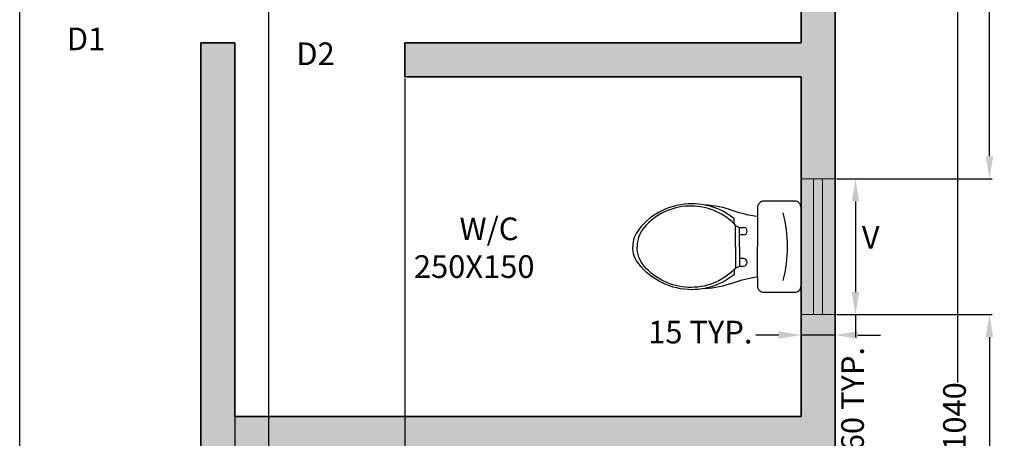
# Model space of a CAD drawing. Units: centimetres. Extents: x 2401 to 3632, y 2122 to 3526.
# Tile 7 of 10: x 2885 to 3320, y 2921 to 3106. Entities that reach past the tile are written whole.
import ezdxf

# ---------------------------------------------------------------- set-up
doc = ezdxf.new("R2010")
doc.units = ezdxf.units.CM
for name, color, linetype, lineweight in [('A-ANNO-DIMS', 9, 'Continuous', 18), ('A-ANNO-TEXT', 9, 'Continuous', 18), ('A-AREA-IDEN', 9, 'Continuous', 25), ('A-FLOR-FIXT', 9, 'Continuous', 18), ('A-GLAZ', 4, 'Continuous', 18), ('A-WALL', 7, 'Continuous', 35)]:
    doc.layers.add(name, color=color, linetype=linetype, lineweight=lineweight)
doc.layers.add('A-GLAZ-PATT', color=251, linetype='Continuous', lineweight=13, true_color=0x636466)
doc.layers.add('A-WALL-PATT', color=18, linetype='Continuous', lineweight=13, true_color=0x000000)
doc.layers.add('WC-Detail_dwgmodels.com', color=251, linetype='Continuous')
doc.layers.add('WC-Outline_dwgmodels.com', color=250, linetype='Continuous')
doc.styles.get("Standard").update_dxf_attribs({"font": 'arial.ttf'})
doc.dimstyles.new('ISO-25', dxfattribs={"dimtxt": 10, "dimasz": 10, "dimexe": 1.25, "dimexo": 0.625, "dimtad": 0, "dimtxsty": 'Standard', "dimcen": 2.5, "dimadec": 0, "dimazin": 0, "dimtfac": 1, "dimtmove": 0, "dimatfit": 3, "dimfxl": 1, "dimarcsym": 0})

# ---------------------------------------------------------------- blocks, each defined once
blk = doc.blocks.new('pan')
at = {"layer": 'WC-Detail_dwgmodels.com'}
for p, q in [((2871.05, 3759.24), (2871.96, 3760.91)), ((2871.96, 3760.91), (2871.96, 3762.74)), ((2875.24, 3760.91), (2871.96, 3760.91)), ((2875.24, 3762.74), (2875.24, 3760.91)), ((2880.5, 3760.91), (2875.24, 3760.91)), ((2880.5, 3760.91), (2885.75, 3760.91)), ((2885.75, 3762.74), (2885.75, 3760.91)), ((2885.75, 3760.91), (2889.03, 3760.91)), ((2889.03, 3760.91), (2889.03, 3762.74)), ((2889.94, 3759.24), (2889.03, 3760.91))]:
    blk.add_line(p, q, dxfattribs=at)
for points in [[(2870.35, 3758.55, 0.434217), (2871.96, 3718.84, 0.182634), (2880.5, 3715.73, 2.693815)], [(2868.08, 3758.55, 0.094048), (2862.86, 3748.73, 0.16845)], [(2870.35, 3758.55), (2868.08, 3758.55, 0.416606)], [(2871.05, 3759.24, 0.008985), (2870.35, 3758.55, 0.182634)], [(2880.5, 3759.24), (2871.05, 3759.24, 0.008985)], [(2880.5, 3759.24), (2889.94, 3759.24, -0.444938)], [(2890.64, 3758.55, -0.434217), (2889.03, 3718.84, -0.182634), (2880.5, 3715.73, -2.693815)], [(2889.94, 3759.24, -0.008985), (2890.64, 3758.55, -0.182634)], [(2890.64, 3758.55), (2892.91, 3758.55, -0.416606)], [(2892.91, 3758.55, -0.105447), (2898.5, 3747.44, -0.16845)], [(2862.86, 3748.73, 0.026594), (2862.08, 3745.66, 0.16845)], [(2898.5, 3747.44, -0.015301), (2898.91, 3745.66, -0.16845)]]:
    blk.add_lwpolyline(points, format="xyb", dxfattribs=at)
for centre, radius, start, end in [((2880.52, 3723.1), 59.08, 90.028, 104.6712), ((2880.47, 3723.1), 59.08, 75.3288, 89.972), ((2873.6, 3762.74), 1.64, 0, 180), ((2887.39, 3762.74), 1.64, 0, 180)]:
    blk.add_arc(centre, radius, start, end, dxfattribs=at)
at = {"layer": 'WC-Outline_dwgmodels.com'}
for points in [[(2897.74, 3768.89, 0.414214), (2900.63, 3771.78), (2900.63, 3785.26, 0.414214), (2897.74, 3788.15), (2880.5, 3788.15), (2863.25, 3788.15, 0.414214), (2860.36, 3785.26), (2860.36, 3771.78, 0.414214), (2863.25, 3768.89), (2867.2, 3768.89, -0.052345), (2864.6, 3758.11, 0.071131), (2862.08, 3745.66, 0.160777)], [(2867.2, 3768.89), (2880.5, 3768.89, 0.414214)], [(2893.79, 3768.89), (2880.5, 3768.89, -0.414214)], [(2898.91, 3745.66, 0.071131), (2896.39, 3758.11, -0.052345), (2893.79, 3768.89), (2897.74, 3768.89, 0.414214)], [(2862.08, 3745.66, 0.048023), (2861.52, 3739.97, 0.16845)], [(2898.91, 3745.66, -0.048023), (2899.47, 3739.97, -0.16845)], [(2861.52, 3739.97, 0.230343), (2872.88, 3716.47, 0.16845), (2880.5, 3713.83, 2.883082)], [(2899.47, 3739.97, -0.230343), (2888.11, 3716.47, -0.16845), (2880.5, 3713.83, -2.883082)]]:
    blk.add_lwpolyline(points, format="xyb", dxfattribs=at)
blk = doc.blocks.new('*D14')
at = {"layer": 'A-ANNO-DIMS', "color": 0, "lineweight": -2, "transparency": 16777216}
for p, q in [((3246.06, 3451.1), (3300.7, 3451.1)), ((3299.45, 3441.1), (3299.45, 2946.17)), ((3299.45, 2421.1), (3299.45, 2916.04)), ((3246.06, 2411.1), (3300.7, 2411.1))]:
    blk.add_line(p, q, dxfattribs=at)
at = {"layer": 'A-ANNO-DIMS', "color": 0, "transparency": 16777216}
for points in [[(3297.79, 3441.1), (3301.12, 3441.1), (3299.45, 3451.1)], [(3297.79, 2421.1), (3301.12, 2421.1), (3299.45, 2411.1)]]:
    blk.add_solid(points, dxfattribs=at)
at = {"layer": 'Defpoints', "color": 0, "transparency": 16777216}
for p in [(3245.44, 3451.1), (3245.44, 2411.1), (3299.45, 2411.1)]:
    blk.add_point(p, dxfattribs=at)
at = {"layer": 'A-ANNO-DIMS', "color": 0, "transparency": 16777216, "insert": (3299.45, 2931.1), "char_height": 10, "attachment_point": 5, "rotation": 90}
blk.add_mtext('1040', dxfattribs=at)
blk = doc.blocks.new('VENT-600')
for p, q in [((15, 60), (0, 60)), ((5.5, 60), (5.5, 0)), ((9.5, 60), (9.5, 0)), ((15, 0), (0, 0))]:
    blk.add_line(p, q)
blk = doc.blocks.new('*D22')
at = {"layer": 'A-ANNO-DIMS', "color": 0, "lineweight": -2, "transparency": 16777216}
for p, q in [((3246.06, 3036.1), (3255.69, 3036.1)), ((3254.44, 3026.1), (3254.44, 2986.1)), ((3246.06, 2976.1), (3255.69, 2976.1)), ((3254.44, 2976.1), (3254.44, 2966.1))]:
    blk.add_line(p, q, dxfattribs=at)
at = {"layer": 'A-ANNO-DIMS', "color": 0, "transparency": 16777216}
for points in [[(3252.77, 3026.1), (3256.1, 3026.1), (3254.44, 3036.1)], [(3252.77, 2986.1), (3256.1, 2986.1), (3254.44, 2976.1)]]:
    blk.add_solid(points, dxfattribs=at)
at = {"layer": 'Defpoints', "color": 0, "transparency": 16777216}
for p in [(3245.44, 3036.1), (3245.44, 2976.1), (3254.44, 2976.1)]:
    blk.add_point(p, dxfattribs=at)
at = {"layer": 'A-ANNO-DIMS', "color": 0, "transparency": 16777216, "insert": (3254.44, 2920.31), "char_height": 10, "attachment_point": 5, "rotation": 90}
blk.add_mtext('VENT 60 TYP.', dxfattribs=at)
blk = doc.blocks.new('*D23')
at = {"layer": 'A-ANNO-DIMS', "color": 0, "lineweight": -2, "transparency": 16777216}
for p, q in [((3230.44, 2975.48), (3230.44, 2965.85)), ((3245.44, 2975.48), (3245.44, 2965.85)), ((3220.44, 2967.1), (3210.44, 2967.1)), ((3245.44, 2967.1), (3230.44, 2967.1)), ((3255.44, 2967.1), (3265.44, 2967.1))]:
    blk.add_line(p, q, dxfattribs=at)
at = {"layer": 'A-ANNO-DIMS', "color": 0, "transparency": 16777216}
for points in [[(3220.44, 2968.77), (3220.44, 2965.44), (3230.44, 2967.1)], [(3255.44, 2968.77), (3255.44, 2965.44), (3245.44, 2967.1)]]:
    blk.add_solid(points, dxfattribs=at)
at = {"layer": 'Defpoints', "color": 0, "transparency": 16777216}
for p in [(3230.44, 2976.1), (3245.44, 2976.1), (3230.44, 2967.1)]:
    blk.add_point(p, dxfattribs=at)
at = {"layer": 'A-ANNO-DIMS', "color": 0, "transparency": 16777216, "insert": (3185.94, 2967.1), "char_height": 10, "attachment_point": 5}
blk.add_mtext('15 TYP.', dxfattribs=at)
blk = doc.blocks.new('*D44')
at = {"layer": 'A-ANNO-DIMS', "color": 0, "lineweight": -2, "transparency": 16777216}
for p, q in [((3246.06, 2976.1), (3314.84, 2976.1)), ((3313.59, 2966.1), (3313.59, 2917.29)), ((3313.59, 2846.1), (3313.59, 2894.92)), ((3246.06, 2836.1), (3314.84, 2836.1))]:
    blk.add_line(p, q, dxfattribs=at)
at = {"layer": 'A-ANNO-DIMS', "color": 0, "transparency": 16777216}
for points in [[(3311.92, 2966.1), (3315.25, 2966.1), (3313.59, 2976.1)], [(3311.92, 2846.1), (3315.25, 2846.1), (3313.59, 2836.1)]]:
    blk.add_solid(points, dxfattribs=at)
at = {"layer": 'Defpoints', "color": 0, "transparency": 16777216}
for p in [(3245.44, 2976.1), (3313.59, 2976.1), (3245.44, 2836.1)]:
    blk.add_point(p, dxfattribs=at)
at = {"layer": 'A-ANNO-DIMS', "color": 0, "transparency": 16777216, "insert": (3313.59, 2906.1), "char_height": 10, "attachment_point": 5, "rotation": 90}
blk.add_mtext('140', dxfattribs=at)
blk = doc.blocks.new('*D45')
at = {"layer": 'A-ANNO-DIMS', "color": 0, "lineweight": -2, "transparency": 16777216}
for p, q in [((3246.06, 3206.1), (3314.84, 3206.1)), ((3313.59, 3196.1), (3313.59, 3132.29)), ((3313.59, 3046.1), (3313.59, 3109.92)), ((3246.06, 3036.1), (3314.84, 3036.1))]:
    blk.add_line(p, q, dxfattribs=at)
at = {"layer": 'A-ANNO-DIMS', "color": 0, "transparency": 16777216}
for points in [[(3311.92, 3196.1), (3315.25, 3196.1), (3313.59, 3206.1)], [(3311.92, 3046.1), (3315.25, 3046.1), (3313.59, 3036.1)]]:
    blk.add_solid(points, dxfattribs=at)
at = {"layer": 'Defpoints', "color": 0, "transparency": 16777216}
for p in [(3245.44, 3206.1), (3313.59, 3206.1), (3245.44, 3036.1)]:
    blk.add_point(p, dxfattribs=at)
at = {"layer": 'A-ANNO-DIMS', "color": 0, "transparency": 16777216, "insert": (3313.59, 3121.1), "char_height": 10, "attachment_point": 5, "rotation": 90}
blk.add_mtext('170', dxfattribs=at)
blk = doc.blocks.new('*D50')
at = {"layer": 'A-ANNO-DIMS', "color": 0, "lineweight": -2, "transparency": 16777216}
for p, q in [((2980.44, 3095.48), (2980.44, 2196.7)), ((3055.44, 3080.48), (3055.44, 2196.7)), ((2990.44, 2197.95), (3010.15, 2197.95)), ((3045.44, 2197.95), (3025.72, 2197.95))]:
    blk.add_line(p, q, dxfattribs=at)
at = {"layer": 'A-ANNO-DIMS', "color": 0, "transparency": 16777216}
for points in [[(2990.44, 2199.62), (2990.44, 2196.29), (2980.44, 2197.95)], [(3045.44, 2199.62), (3045.44, 2196.29), (3055.44, 2197.95)]]:
    blk.add_solid(points, dxfattribs=at)
at = {"layer": 'Defpoints', "color": 0, "transparency": 16777216}
for p in [(2980.44, 3096.1), (3055.44, 3081.1), (3055.44, 2197.95)]:
    blk.add_point(p, dxfattribs=at)
at = {"layer": 'A-ANNO-DIMS', "color": 0, "transparency": 16777216, "insert": (3017.94, 2197.95), "char_height": 10, "attachment_point": 5}
blk.add_mtext('75', dxfattribs=at)
blk = doc.blocks.new('*D52')
at = {"layer": 'A-ANNO-DIMS', "color": 0, "lineweight": -2, "transparency": 16777216}
for p, q in [((2885.44, 2411.73), (2885.44, 3520.5)), ((2895.44, 3519.25), (2929.25, 3519.25)), ((2985.44, 3519.25), (2951.62, 3519.25)), ((2995.44, 2591.73), (2995.44, 3520.5))]:
    blk.add_line(p, q, dxfattribs=at)
at = {"layer": 'A-ANNO-DIMS', "color": 0, "transparency": 16777216}
for points in [[(2895.44, 3520.92), (2895.44, 3517.59), (2885.44, 3519.25)], [(2985.44, 3520.92), (2985.44, 3517.59), (2995.44, 3519.25)]]:
    blk.add_solid(points, dxfattribs=at)
at = {"layer": 'Defpoints', "color": 0, "transparency": 16777216}
for p in [(2995.44, 3519.25), (2995.44, 2591.1), (2885.44, 2411.1)]:
    blk.add_point(p, dxfattribs=at)
at = {"layer": 'A-ANNO-DIMS', "color": 0, "transparency": 16777216, "insert": (2940.44, 3519.25), "char_height": 10, "attachment_point": 5}
blk.add_mtext('110', dxfattribs=at)

msp = doc.modelspace()

# ---------------------------------------------------------------- hatches: boundary and pattern name
at = {"layer": 'A-GLAZ-PATT'}
h = msp.add_hatch(color=256, dxfattribs=at)
h.dxf.hatch_style = 1
h.paths.add_polyline_path([(2505.936, 3356.104), (2500.436, 3356.104), (2500.436, 3301.104), (2505.936, 3301.104)])
h.paths.add_polyline_path([(2509.936, 3356.104), (2505.936, 3356.104), (2505.936, 3301.104), (2509.936, 3301.104)])
h.paths.add_polyline_path([(2515.436, 3335.674), (2515.436, 3356.104), (2509.936, 3356.104), (2509.936, 3301.104), (2515.436, 3301.104)])
h.paths.add_polyline_path([(2509.936, 3301.104), (2505.936, 3301.104), (2505.936, 3261.104), (2509.936, 3261.104)])
h.paths.add_polyline_path([(2515.436, 3301.104), (2509.936, 3301.104), (2509.936, 3261.104), (2515.436, 3261.104)])
h.paths.add_polyline_path([(2505.936, 3301.104), (2500.436, 3301.104), (2500.436, 3261.104), (2505.936, 3261.104)])
h.paths.add_polyline_path([(2515.436, 3261.104), (2509.936, 3261.104), (2509.936, 3206.104), (2515.436, 3206.104)])
h.paths.add_polyline_path([(2505.936, 3261.104), (2500.436, 3261.104), (2500.436, 3206.104), (2505.936, 3206.104)])
h.paths.add_polyline_path([(2509.936, 3261.104), (2505.936, 3261.104), (2505.936, 3206.104), (2509.936, 3206.104)])
h.paths.add_polyline_path([(3127.936, 3451.104), (3072.936, 3451.104), (3072.936, 3445.604), (3127.936, 3445.604)])
h.paths.add_polyline_path([(3032.936, 3441.604), (2977.936, 3441.604), (2977.936, 3436.104), (3032.936, 3436.104)])
h.paths.add_polyline_path([(3032.936, 3451.104), (2977.936, 3451.104), (2977.936, 3445.604), (3032.936, 3445.604)])
h.paths.add_polyline_path([(3032.936, 3445.604), (2977.936, 3445.604), (2977.936, 3441.604), (3032.936, 3441.604)])
h.paths.add_polyline_path([(3072.936, 3451.104), (3032.936, 3451.104), (3032.936, 3445.604), (3072.936, 3445.604)])
h.paths.add_polyline_path([(3072.936, 3445.604), (3032.936, 3445.604), (3032.936, 3441.604), (3072.936, 3441.604)])
h.paths.add_polyline_path([(3072.936, 3441.604), (3032.936, 3441.604), (3032.936, 3436.104), (3072.936, 3436.104)])
h.paths.add_polyline_path([(3127.936, 3441.604), (3072.936, 3441.604), (3072.936, 3436.104), (3127.936, 3436.104)])
h.paths.add_polyline_path([(3127.936, 3445.604), (3072.936, 3445.604), (3072.936, 3441.604), (3127.936, 3441.604)])
h.paths.add_polyline_path([(3245.436, 3356.104), (3239.936, 3356.104), (3239.936, 3301.104), (3245.436, 3301.104)])
h.paths.add_polyline_path([(3239.936, 3356.104), (3235.936, 3356.104), (3235.936, 3301.104), (3239.936, 3301.104)])
h.paths.add_polyline_path([(3235.936, 3356.104), (3230.436, 3356.104), (3230.436, 3301.104), (3235.936, 3301.104)])
h.paths.add_polyline_path([(3235.936, 3301.104), (3230.436, 3301.104), (3230.436, 3261.104), (3235.936, 3261.104)])
h.paths.add_polyline_path([(3239.936, 3301.104), (3235.936, 3301.104), (3235.936, 3261.104), (3239.936, 3261.104)])
h.paths.add_polyline_path([(3245.436, 3301.104), (3239.936, 3301.104), (3239.936, 3261.104), (3245.436, 3261.104)])
h.paths.add_polyline_path([(3245.436, 3261.104), (3239.936, 3261.104), (3239.936, 3206.104), (3245.436, 3206.104)])
h.paths.add_polyline_path([(3239.936, 3261.104), (3235.936, 3261.104), (3235.936, 3206.104), (3239.936, 3206.104)])
h.paths.add_polyline_path([(3235.936, 3261.104), (3230.436, 3261.104), (3230.436, 3206.104), (3235.936, 3206.104)])
h.paths.add_polyline_path([(3239.936, 3036.104), (3235.936, 3036.104), (3235.936, 2976.104), (3239.936, 2976.104)])
h.paths.add_polyline_path([(3235.936, 3036.104), (3230.436, 3036.104), (3230.436, 2976.104), (3235.936, 2976.104)])
h.paths.add_polyline_path([(3245.436, 3036.104), (3239.936, 3036.104), (3239.936, 2976.104), (3245.436, 2976.104)])
h.paths.add_polyline_path([(3235.936, 2836.104), (3230.436, 2836.104), (3230.436, 2781.104), (3235.936, 2781.104)])
h.paths.add_polyline_path([(3245.436, 2836.104), (3239.936, 2836.104), (3239.936, 2781.104), (3245.436, 2781.104)])
h.paths.add_polyline_path([(3239.936, 2836.104), (3235.936, 2836.104), (3235.936, 2781.104), (3239.936, 2781.104)])
h.paths.add_polyline_path([(3245.436, 2781.104), (3239.936, 2781.104), (3239.936, 2741.104), (3245.436, 2741.104)])
h.paths.add_polyline_path([(3239.936, 2781.104), (3235.936, 2781.104), (3235.936, 2741.104), (3239.936, 2741.104)])
h.paths.add_polyline_path([(3235.936, 2781.104), (3230.436, 2781.104), (3230.436, 2741.104), (3235.936, 2741.104)])
h.paths.add_polyline_path([(3245.436, 2741.104), (3239.936, 2741.104), (3239.936, 2686.104), (3245.436, 2686.104)])
h.paths.add_polyline_path([(3239.936, 2741.104), (3235.936, 2741.104), (3235.936, 2686.104), (3239.936, 2686.104)])
h.paths.add_polyline_path([(3235.936, 2741.104), (3230.436, 2741.104), (3230.436, 2686.104), (3235.936, 2686.104)])
h.paths.add_polyline_path([(3187.936, 2606.104), (3132.936, 2606.104), (3132.936, 2600.604), (3187.936, 2600.604)])
h.paths.add_polyline_path([(3187.936, 2600.604), (3132.936, 2600.604), (3132.936, 2596.604), (3187.936, 2596.604)])
h.paths.add_polyline_path([(3187.936, 2596.604), (3132.936, 2596.604), (3132.936, 2591.104), (3187.936, 2591.104)])
h.paths.add_polyline_path([(3132.936, 2596.604), (3092.936, 2596.604), (3092.936, 2591.104), (3132.936, 2591.104)])
h.paths.add_polyline_path([(3132.936, 2600.604), (3092.936, 2600.604), (3092.936, 2596.604), (3132.936, 2596.604)])
h.paths.add_polyline_path([(3132.936, 2606.104), (3092.936, 2606.104), (3092.936, 2600.604), (3132.936, 2600.604)])
h.paths.add_polyline_path([(3092.936, 2596.604), (3037.936, 2596.604), (3037.936, 2591.104), (3092.936, 2591.104)])
h.paths.add_polyline_path([(3092.936, 2600.604), (3037.936, 2600.604), (3037.936, 2596.604), (3092.936, 2596.604)])
h.paths.add_polyline_path([(3092.936, 2606.104), (3037.936, 2606.104), (3037.936, 2600.604), (3092.936, 2600.604)])
h.paths.add_polyline_path([(2803.613, 3432.66), (2826.471, 3432.66), (2826.471, 3453.267), (2803.613, 3453.267)], flags=9)
h.paths.add_polyline_path([(2904.038, 3087.418), (2926.896, 3087.418), (2926.896, 3108.025), (2904.038, 3108.025)], flags=9)
h.paths.add_polyline_path([(2801.908, 3105.391), (2824.766, 3105.391), (2824.766, 3125.998), (2801.908, 3125.998)], flags=9)
h.paths.add_polyline_path([(2757.576, 2660.284), (2780.434, 2660.284), (2780.434, 2680.892), (2757.576, 2680.892)], flags=9)
h.paths.add_polyline_path([(3004.446, 3080.825), (3027.304, 3080.825), (3027.304, 3101.432), (3004.446, 3101.432)], flags=9)
h.paths.add_polyline_path([(2805.63, 2777.019), (2828.489, 2777.019), (2828.489, 2797.626), (2805.63, 2797.626)], flags=9)
h.paths.add_polyline_path([(3094.334, 2572.754), (3128.823, 2572.754), (3128.823, 2593.361), (3094.334, 2593.361)], flags=9)
h.paths.add_polyline_path([(2931.792, 2588.154), (2946.88, 2588.154), (2946.88, 2608.761), (2931.792, 2608.761)], flags=9)
h.paths.add_polyline_path([(2582.951, 2415.87), (2664.015, 2415.87), (2664.015, 2453.184), (2582.951, 2453.184)], flags=9)
h.paths.add_polyline_path([(2622.234, 2685.113), (2683.168, 2685.113), (2683.168, 2722.427), (2622.234, 2722.427)], flags=9)
h.paths.add_polyline_path([(3027.646, 2511.408), (3088.58, 2511.408), (3088.58, 2548.722), (3027.646, 2548.722)], flags=9)
h.paths.add_polyline_path([(3020.004, 2720.966), (3092.521, 2720.966), (3092.521, 2758.281), (3020.004, 2758.281)], flags=9)
h.paths.add_polyline_path([(2628.506, 2930.416), (2689.441, 2930.416), (2689.441, 2967.73), (2628.506, 2967.73)], flags=9)
h.paths.add_polyline_path([(3056.573, 2986.666), (3117.507, 2986.666), (3117.507, 3023.981), (3056.573, 3023.981)], flags=9)
h.paths.add_polyline_path([(3083.425, 3281.357), (3164.489, 3281.357), (3164.489, 3318.672), (3083.425, 3318.672)], flags=9)
h.paths.add_polyline_path([(2658.367, 3249.15), (2724.683, 3249.15), (2724.683, 3286.465), (2658.367, 3286.465)], flags=9)
at = {"layer": 'A-WALL-PATT'}
h = msp.add_hatch(color=256, dxfattribs=at)
h.dxf.hatch_style = 1
h.paths.add_polyline_path([(2765.436, 3451.104), (2500.436, 3451.104), (2500.436, 3356.104), (2515.436, 3356.104), (2515.436, 3436.104), (2765.436, 3436.104)])
h.paths.add_polyline_path([(3245.436, 3451.104), (3127.936, 3451.104), (3127.936, 3436.104), (3185.226, 3436.104), (3185.226, 3436.735), (3230.436, 3436.735), (3230.436, 3356.104), (3245.436, 3356.104)])
h.paths.add_polyline_path([(3245.436, 2686.104), (3230.436, 2686.104), (3230.436, 2606.104), (3187.936, 2606.104), (3187.936, 2591.104), (3245.436, 2591.104)])
h.paths.add_polyline_path([(3037.936, 2606.104), (2995.436, 2606.104), (2995.436, 2591.104), (3037.936, 2591.104)])
h.paths.add_polyline_path([(3245.436, 2976.104), (3230.436, 2976.104), (3230.436, 2931.104), (2980.436, 2931.104), (2980.436, 3096.104), (2965.436, 3096.104), (2965.436, 2916.104), (3230.436, 2916.104), (3230.436, 2836.104), (3245.436, 2836.104)])
h.paths.add_polyline_path([(3230.436, 3096.104), (3055.436, 3096.104), (3055.436, 3081.104), (3230.436, 3081.104)], flags=17)
h.paths.add_polyline_path([(2977.936, 3451.104), (2860.436, 3451.104), (2860.436, 3096.104), (2875.436, 3096.104), (2875.436, 3436.104), (2977.936, 3436.104)])
h.paths.add_polyline_path([(2765.436, 3126.104), (2515.436, 3126.104), (2515.436, 3206.104), (2500.436, 3206.104), (2500.436, 3028.604), (2515.436, 3028.604), (2515.436, 3111.104), (2765.436, 3111.104)])
h.paths.add_polyline_path([(2780.436, 2796.104), (2515.436, 2796.104), (2515.436, 2878.604), (2500.436, 2878.604), (2500.436, 2736.104), (2515.436, 2736.104), (2515.436, 2781.104), (2765.436, 2781.104), (2765.436, 2706.104), (2780.436, 2706.104)])
h.paths.add_polyline_path([(2780.436, 2631.104), (2515.436, 2631.104), (2515.436, 2676.104), (2500.436, 2676.104), (2500.436, 2523.604), (2515.436, 2523.604), (2515.436, 2616.104), (2780.436, 2616.104)])
h.paths.add_polyline_path([(2885.436, 2796.104), (2870.436, 2796.104), (2870.436, 2281.104), (2762.936, 2281.104), (2762.936, 2266.104), (2885.436, 2266.104)])
h.paths.add_polyline_path([(2612.936, 2281.104), (2515.436, 2281.104), (2515.436, 2373.604), (2500.436, 2373.604), (2500.436, 2266.104), (2612.936, 2266.104)])
h = msp.add_hatch(color=256, dxfattribs=at)
h.dxf.hatch_style = 1
h.paths.add_polyline_path([(3245.436, 3206.104), (3230.436, 3206.104), (3230.436, 3165.474), (3230.436, 3096.104), (3055.436, 3096.104), (3055.436, 3081.104), (3230.436, 3081.104), (3230.436, 3036.104), (3245.436, 3036.104)])

# ---------------------------------------------------------------- linework, layer by layer
at = {"layer": 'A-WALL'}
for p, q in [((3230.436, 3096.104), (3230.436, 3436.104)), ((2965.436, 2916.104), (2965.436, 3096.104)), ((2980.436, 3096.104), (2965.436, 3096.104)), ((2980.436, 2931.104), (2980.436, 3096.104)), ((3230.436, 3096.104), (3055.436, 3096.104)), ((3055.436, 3081.104), (3055.436, 3096.104)), ((3230.436, 3081.104), (3055.436, 3081.104)), ((3230.436, 2931.104), (3230.436, 3081.104)), ((3230.436, 2931.104), (2980.436, 2931.104))]:
    msp.add_line(p, q, dxfattribs=at)
msp.add_lwpolyline([(2885.436, 2411.104), (3245.436, 2411.104), (3245.436, 3451.104), (2860.436, 3451.104)], dxfattribs=at)

# ---------------------------------------------------------------- block references
at = {"layer": 'A-FLOR-FIXT', "rotation": 270}
msp.add_blockref('pan', (-557.715, 5886.6), dxfattribs=at)
at = {"layer": 'A-GLAZ', "rotation": 180}
msp.add_blockref('VENT-600', (3245.436, 3036.104), dxfattribs=at)

# ---------------------------------------------------------------- texts
at = {"layer": 'A-ANNO-TEXT', "char_height": 10, "attachment_point": 1}
for s, width, insert in [('\\pxqc;D1', 66.28614, (2881.581, 3102.919)), ('\\pxqc;D2', 51.84914, (2990.121, 3096.327)), ('\\pxqc;V', 66.28614, (3228.006, 3015.281))]:
    msp.add_mtext_dynamic_manual_height_columns(s, width=width, gutter_width=12.5, heights=[0], dxfattribs=dict(at, insert=insert))
at = {"layer": 'A-AREA-IDEN', "insert": (3059.482, 3019.005), "char_height": 10, "attachment_point": 1}
msp.add_mtext_dynamic_manual_height_columns('\\pxqc;W/C\\P\\pq*;250X150', width=66.28614, gutter_width=12.5, heights=[0], dxfattribs=at)

# ---------------------------------------------------------------- dimensions: what is measured, and where the dimension line sits
at = {"layer": 'A-ANNO-DIMS'}
for base, p1, p2, picture, middle in [((2995.436, 3519.254), (2885.436, 2411.104), (2995.436, 2591.104), '*D52', (2940.436, 3519.254)), ((3055.436, 2197.954), (2980.436, 3096.104), (3055.436, 3081.104), '*D50', (3017.936, 2197.954))]:
    dim = msp.add_linear_dim(base=base, p1=p1, p2=p2, dimstyle='ISO-25', override={"dimdec": 0, "dimlfac": 1, "dimrnd": 0, "dimzin": 0, "dimdsep": 46, "dimlunit": 2}, dxfattribs=at)
    dim.commit()
    dim.dimension.update_dxf_attribs({"geometry": picture, "text_midpoint": middle})
for base, p1, p2, override, picture, middle in [((3299.454, 2411.104), (3245.436, 3451.104), (3245.436, 2411.104), {"dimclrd": 0, "dimclre": 0, "dimclrt": 0}, '*D14', (3299.454, 2931.104)), ((3313.586, 3206.104), (3245.436, 3036.104), (3245.436, 3206.104), {"dimdec": 0, "dimlfac": 1, "dimrnd": 0, "dimzin": 0, "dimdsep": 46, "dimlunit": 2}, '*D45', (3313.586, 3121.104)), ((3313.586, 2976.104), (3245.436, 2836.104), (3245.436, 2976.104), {"dimdec": 0, "dimlfac": 1, "dimrnd": 0, "dimzin": 0, "dimdsep": 46, "dimlunit": 2}, '*D44', (3313.586, 2906.104))]:
    dim = msp.add_linear_dim(base=base, p1=p1, p2=p2, angle=90, dimstyle='ISO-25', override=override, dxfattribs=at)
    dim.commit()
    dim.dimension.update_dxf_attribs({"geometry": picture, "text_midpoint": middle})
for base, p1, p2, angle, text, picture, middle in [((3254.436, 2976.104), (3245.436, 3036.104), (3245.436, 2976.104), 270, 'VENT <> TYP.', '*D22', (3254.436, 2920.312)), ((3230.436, 2967.104), (3245.436, 2976.104), (3230.436, 2976.104), 180, '<> TYP.', '*D23', (3185.943, 2967.104))]:
    dim = msp.add_linear_dim(base=base, p1=p1, p2=p2, angle=angle, text=text, dimstyle='ISO-25', override={"dimdec": 0, "dimlfac": 1, "dimrnd": 0, "dimzin": 0, "dimdsep": 46, "dimlunit": 2}, dxfattribs=at)
    dim.commit()
    dim.dimension.update_dxf_attribs({"geometry": picture, "text_midpoint": middle})

doc.saveas('drawing.dxf')
